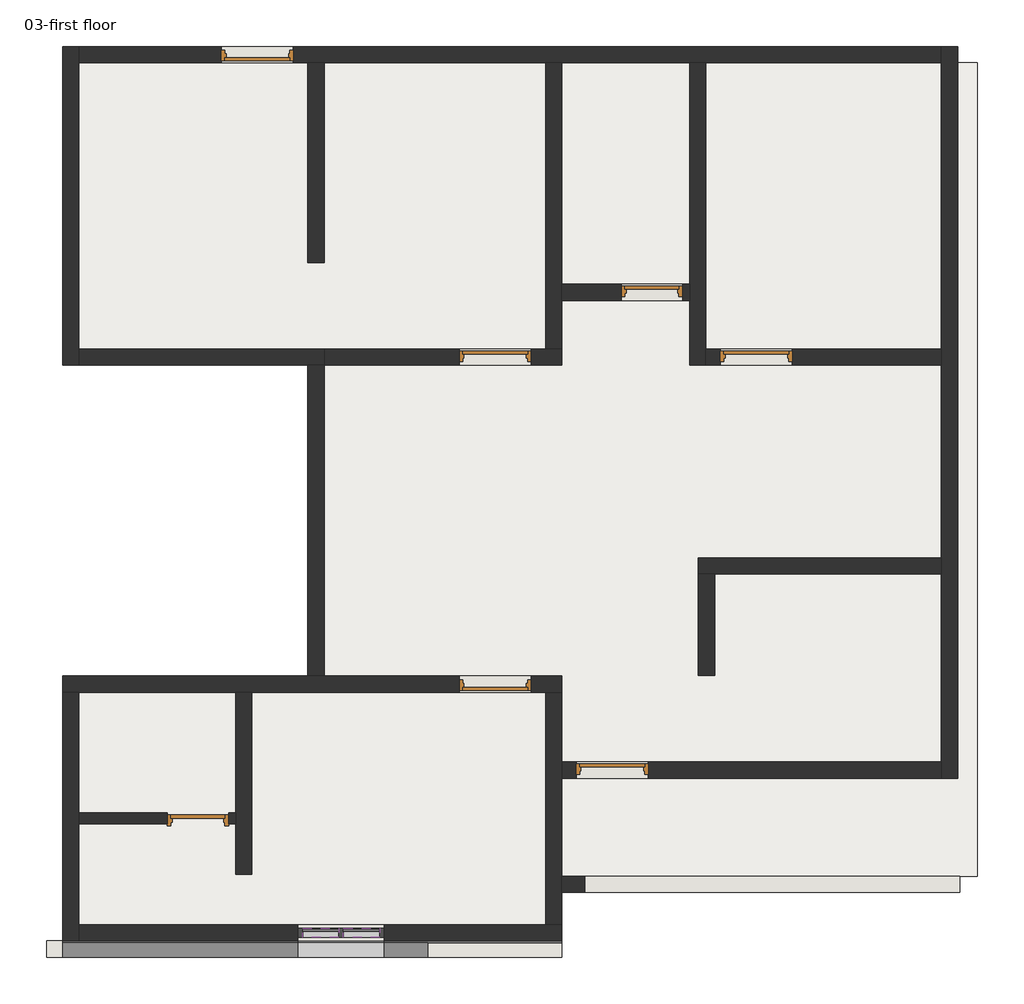
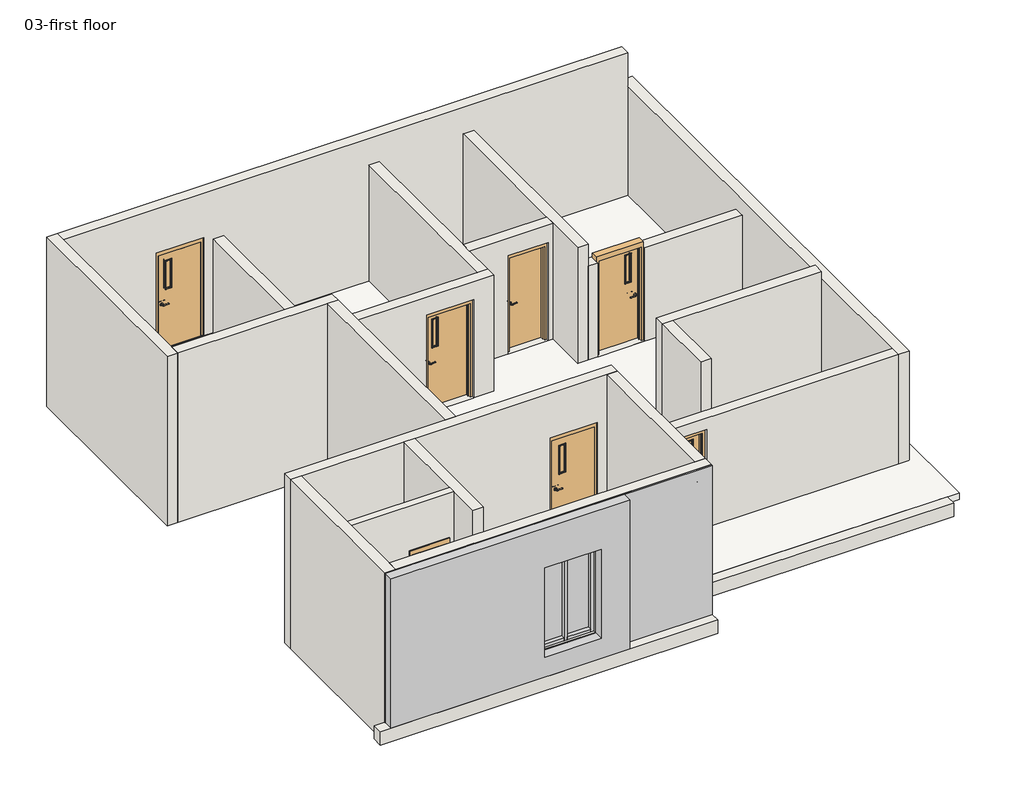
# One storey, incomplete: 23 walls, 7 doors, 7 members, 2 plates, 1 furniture element, 1 slab.
"""IFC4 building model written with IfcOpenShell, lengths in millimetres."""

from ifc_helpers import new_model, si_unit, frame, origin, place, context, project, spatial, polyline, outline, extrude, faceted_brep, transform, mapped, element, save
from components import m_door_passage_single_flush_750_x_2000mm_a9826c90, m_door_passage_single_flush_750_x_2000mm_58848773, m_door_passage_single_vision_lite_900_x_2100_f7eb172f, m_door_passage_single_vision_lite_900_x_2100_15962226, casework_2_casework_2_9c5fcee0, rectangular_mullion_65_x_125mm_rectangular_623ff0e3, rectangular_mullion_65_x_125mm_rectangular_d57ab73f, rectangular_mullion_65_x_125mm_rectangular_2_b62c991d, system_panel_glazed_9cdd2f26

model = new_model("IFC4")

# Units and contexts
model_context = context("Model", 3, world=origin())
ifc_project = project(units=[si_unit("LENGTHUNIT", "METRE", prefix="MILLI")], contexts=[model_context])

# Site, building, storey
site = spatial("IfcSite", under=ifc_project)
building = spatial("IfcBuilding", under=site)
storey = spatial("IfcBuildingStorey", under=building, Name="03-first floor", Elevation=3800.0)

# Doors
placement = place(None, origin())
m_door_passage_single_flush_750_x_2000mm_shape = m_door_passage_single_flush_750_x_2000mm_a9826c90(model_context)
element("IfcDoor", 1, ObjectType="M_Door-Passage-Single-Flush : 750 x 2000mm", at=placement, inside=storey, context=model_context, shape_type="MappedRepresentation", body=[
    mapped(m_door_passage_single_flush_750_x_2000mm_shape, transform((-18812.7520625, -8532.3980844, 4400.0), x_axis=(1.0, 0.0, 0.0), y_axis=(0.0, 1.0, 0.0), z_axis=(0.0, 0.0, 1.0))),
])
m_door_passage_single_flush_750_x_2000mm_2_shape = m_door_passage_single_flush_750_x_2000mm_58848773(model_context)
element("IfcDoor", 2, ObjectType="M_Door-Passage-Single-Flush : 750 x 2000mm", at=placement, inside=storey, context=model_context, shape_type="MappedRepresentation", body=[
    mapped(m_door_passage_single_flush_750_x_2000mm_2_shape, transform((-12512.7520625, -1227.8980844, 4400.0), x_axis=(1.0, 0.0, 0.0), y_axis=(0.0, 1.0, 0.0), z_axis=(0.0, 0.0, 1.0))),
])
m_door_passage_single_vision_lite_900_x_2100_shape = m_door_passage_single_vision_lite_900_x_2100_f7eb172f(model_context)
element("IfcDoor", 3, ObjectType="M_Door-Passage-Single-Vision_Lite : 900 x 2100", at=placement, inside=storey, context=model_context, shape_type="MappedRepresentation", body=[
    mapped(m_door_passage_single_vision_lite_900_x_2100_shape, transform((-13062.7520625, -7859.8980844, 4400.0), x_axis=(-1.0, 0.0, 0.0), y_axis=(0.0, -1.0, 0.0), z_axis=(0.0, 0.0, 1.0))),
])
element("IfcDoor", 4, ObjectType="M_Door-Passage-Single-Vision_Lite : 900 x 2100", at=placement, inside=storey, context=model_context, shape_type="MappedRepresentation", body=[
    mapped(m_door_passage_single_vision_lite_900_x_2100_shape, transform((-11062.7520625, -2127.8980844, 4400.0), x_axis=(-1.0, 0.0, 0.0), y_axis=(0.0, -1.0, 0.0), z_axis=(0.0, 0.0, 1.0))),
])
element("IfcDoor", 5, ObjectType="M_Door-Passage-Single-Vision_Lite : 900 x 2100", at=placement, inside=storey, context=model_context, shape_type="MappedRepresentation", body=[
    mapped(m_door_passage_single_vision_lite_900_x_2100_shape, transform((-14687.7520625, -6655.1980844, 4400.0), x_axis=(1.0, 0.0, 0.0), y_axis=(0.0, 1.0, 0.0), z_axis=(0.0, 0.0, 1.0))),
])
element("IfcDoor", 6, ObjectType="M_Door-Passage-Single-Vision_Lite : 900 x 2100", at=placement, inside=storey, context=model_context, shape_type="MappedRepresentation", body=[
    mapped(m_door_passage_single_vision_lite_900_x_2100_shape, transform((-17987.7520625, 2084.8019156, 4400.0), x_axis=(1.0, 0.0, 0.0), y_axis=(0.0, 1.0, 0.0), z_axis=(0.0, 0.0, 1.0))),
])
m_door_passage_single_vision_lite_900_x_2100_2_shape = m_door_passage_single_vision_lite_900_x_2100_15962226(model_context)
element("IfcDoor", 7, ObjectType="M_Door-Passage-Single-Vision_Lite : 900 x 2100", at=placement, inside=storey, context=model_context, shape_type="MappedRepresentation", body=[
    mapped(m_door_passage_single_vision_lite_900_x_2100_2_shape, transform((-14687.7520625, -2127.8980844, 4400.0), x_axis=(1.0, 0.0, 0.0), y_axis=(0.0, 1.0, 0.0), z_axis=(0.0, 0.0, 1.0))),
])

# Furniture
casework_2_casework_2_shape = casework_2_casework_2_9c5fcee0(model_context)
element("IfcFurniture", 8, ObjectType="Casework 2 : Casework 2", at=placement, inside=storey, context=model_context, shape_type="MappedRepresentation", body=[
    mapped(casework_2_casework_2_shape, transform((0.0, 0.0, 0.0), x_axis=(1.0, 0.0, 0.0), y_axis=(0.0, 1.0, 0.0), z_axis=(0.0, 0.0, 1.0))),
])

# Members
rectangular_mullion_65_x_125mm_rectangular_shape = rectangular_mullion_65_x_125mm_rectangular_623ff0e3(model_context)
element("IfcMember", 9, ObjectType="Rectangular Mullion : 65 x 125mm rectangular", at=placement, inside=storey, context=model_context, shape_type="MappedRepresentation", body=[
    mapped(rectangular_mullion_65_x_125mm_rectangular_shape, transform((-16290.2520625, -10113.5480844, 6700.0), x_axis=(0.0, 0.0, 1.0), y_axis=(0.0, -1.0, 0.0), z_axis=(1.0, 0.0, 0.0))),
])
element("IfcMember", 10, ObjectType="Rectangular Mullion : 65 x 125mm rectangular", at=placement, inside=storey, context=model_context, shape_type="MappedRepresentation", body=[
    mapped(rectangular_mullion_65_x_125mm_rectangular_shape, transform((-16857.7520625, -10113.5480844, 6700.0), x_axis=(0.0, 0.0, 1.0), y_axis=(0.0, -1.0, 0.0), z_axis=(1.0, 0.0, 0.0))),
])
element("IfcMember", 11, ObjectType="Rectangular Mullion : 65 x 125mm rectangular", at=placement, inside=storey, context=model_context, shape_type="MappedRepresentation", body=[
    mapped(rectangular_mullion_65_x_125mm_rectangular_shape, transform((-17360.2520625, -10113.5480844, 4700.0), x_axis=(0.0, 0.0, -1.0), y_axis=(0.0, -1.0, 0.0), z_axis=(-1.0, 0.0, 0.0))),
])
element("IfcMember", 12, ObjectType="Rectangular Mullion : 65 x 125mm rectangular", at=placement, inside=storey, context=model_context, shape_type="MappedRepresentation", body=[
    mapped(rectangular_mullion_65_x_125mm_rectangular_shape, transform((-16792.7520625, -10113.5480844, 4700.0), x_axis=(0.0, 0.0, -1.0), y_axis=(0.0, -1.0, 0.0), z_axis=(-1.0, 0.0, 0.0))),
])
rectangular_mullion_65_x_125mm_rectangular_2_shape = rectangular_mullion_65_x_125mm_rectangular_d57ab73f(model_context)
element("IfcMember", 13, ObjectType="Rectangular Mullion : 65 x 125mm rectangular", at=placement, inside=storey, context=model_context, shape_type="MappedRepresentation", body=[
    mapped(rectangular_mullion_65_x_125mm_rectangular_2_shape, transform((-16225.2520625, -10113.5480844, 4700.0), x_axis=(1.0, 0.0, 0.0), y_axis=(0.0, -1.0, 0.0), z_axis=(0.0, 0.0, -1.0))),
])
element("IfcMember", 14, ObjectType="Rectangular Mullion : 65 x 125mm rectangular", at=placement, inside=storey, context=model_context, shape_type="MappedRepresentation", body=[
    mapped(rectangular_mullion_65_x_125mm_rectangular_2_shape, transform((-17425.2520625, -10113.5480844, 6700.0), x_axis=(-1.0, 0.0, 0.0), y_axis=(0.0, -1.0, 0.0), z_axis=(0.0, 0.0, 1.0))),
])
rectangular_mullion_65_x_125mm_rectangular_2_2_shape = rectangular_mullion_65_x_125mm_rectangular_2_b62c991d(model_context)
element("IfcMember", 15, ObjectType="Rectangular Mullion : 65 x 125mm rectangular 2", at=placement, inside=storey, context=model_context, shape_type="MappedRepresentation", body=[
    mapped(rectangular_mullion_65_x_125mm_rectangular_2_2_shape, transform((-16825.2520625, -10113.5480844, 4700.0), x_axis=(1.0, 0.0, 0.0), y_axis=(0.0, -1.0, 0.0), z_axis=(0.0, 0.0, -1.0))),
])

# Plates
system_panel_glazed_shape = system_panel_glazed_9cdd2f26(model_context)
element("IfcPlate", 16, ObjectType="System Panel : Glazed", at=placement, inside=storey, context=model_context, shape_type="MappedRepresentation", body=[
    mapped(system_panel_glazed_shape, transform((-17109.0020625, -10113.5480844, 4765.0), x_axis=(1.0, 0.0, 0.0), y_axis=(0.0, 1.0, 0.0), z_axis=(0.0, 0.0, 1.0))),
])
element("IfcPlate", 17, ObjectType="System Panel : Glazed", at=placement, inside=storey, context=model_context, shape_type="MappedRepresentation", body=[
    mapped(system_panel_glazed_shape, transform((-16541.5020625, -10113.5480844, 4765.0), x_axis=(1.0, 0.0, 0.0), y_axis=(0.0, 1.0, 0.0), z_axis=(0.0, 0.0, 1.0))),
])

# Slab
element("IfcSlab", 18, ObjectType="01-150 floor", at=placement, inside=storey, context=model_context, shape_type="SweptSolid", body=[
    extrude(outline(polyline([(-7995.7520625, 1965.9519156), (-7995.7520625, -9326.0480844), (-9470.7520625, -9326.0480844), (-13987.7520625, -9326.0480844), (-13987.7520625, -10001.0480844), (-20462.7520625, -10001.0480844), (-20462.7520625, -6774.0480844), (-17062.7520625, -6774.0480844), (-17062.7520625, -2009.0480844), (-20462.7520625, -2009.0480844), (-20462.7520625, 1965.9519156), (-7995.7520625, 1965.9519156)])), frame((0.0, 0.0, 4250.0), z_axis=(0.0, 0.0, 1.0), x_axis=(1.0, 0.0, 0.0)), (0.0, 0.0, 1.0), 150.0),
])

# Walls
element("IfcWall", 19, ObjectType="01-225 wall", at=placement, inside=storey, context=model_context, shape_type="Brep", body=[
    faceted_brep([(-20687.7520625, 2190.9519156, 3800.0), (-20687.7520625, -2234.0480844, 3800.0), (-20687.7520625, -2234.0480844, 7600.0), (-20687.7520625, 2190.9519156, 7600.0), (-20462.7520625, 2190.9519156, 3800.0), (-20462.7520625, 2190.9519156, 7600.0), (-20462.7520625, 1965.9519156, 7600.0), (-20462.7520625, -2009.0480844, 7600.0), (-20462.7520625, -2234.0480844, 7600.0), (-20462.7520625, -2234.0480844, 3800.0), (-20462.7520625, -2009.0480844, 3800.0), (-20462.7520625, 1965.9519156, 3800.0)], [[[0, 1, 2, 3]], [[4, 5, 6, 7, 8, 9, 10, 11]], [[1, 0, 4, 11, 10, 9]], [[3, 2, 8, 7, 6, 5]], [[0, 3, 5, 4]], [[2, 1, 9, 8]]]),
])
element("IfcWall", 20, ObjectType="01-225 wall", at=placement, inside=storey, context=model_context, shape_type="Brep", body=[
    faceted_brep([(-20462.7520625, -10226.0480844, 3800.0), (-13762.7520625, -10226.0480844, 3800.0), (-13762.7520625, -10226.0480844, 7600.0), (-20462.7520625, -10226.0480844, 7600.0), (-17425.2520625, -10226.0480844, 4700.0), (-17425.2520625, -10226.0480844, 6700.0), (-16225.2520625, -10226.0480844, 6700.0), (-16225.2520625, -10226.0480844, 4700.0), (-13762.7520625, -10001.0480844, 3800.0), (-13987.7520625, -10001.0480844, 3800.0), (-20462.7520625, -10001.0480844, 3800.0), (-20462.7520625, -10001.0480844, 7600.0), (-13987.7520625, -10001.0480844, 7600.0), (-13762.7520625, -10001.0480844, 7600.0), (-17425.2520625, -10001.0480844, 6700.0), (-17425.2520625, -10001.0480844, 4700.0), (-16225.2520625, -10001.0480844, 4700.0), (-16225.2520625, -10001.0480844, 6700.0)], [[[0, 1, 2, 3], [4, 5, 6, 7]], [[8, 9, 10, 11, 12, 13], [14, 15, 16, 17]], [[1, 0, 10, 9, 8]], [[3, 2, 13, 12, 11]], [[4, 15, 14, 5]], [[5, 14, 17, 6]], [[6, 17, 16, 7]], [[15, 4, 7, 16]], [[1, 8, 13, 2]], [[3, 11, 10, 0]]]),
])
element("IfcWall", 21, ObjectType="01-225 wall", at=placement, inside=storey, context=model_context, shape_type="Brep", body=[
    faceted_brep([(-8270.7520625, -7966.0480844, 3800.0), (-8270.7520625, 2190.9519156, 3800.0), (-8270.7520625, 2190.9519156, 6850.0), (-8270.7520625, -7966.0480844, 6850.0), (-8495.7520625, -7966.0480844, 3800.0), (-8495.7520625, -7966.0480844, 6850.0), (-8495.7520625, -7741.0480844, 6850.0), (-8495.7520625, 2190.9519156, 6850.0), (-8495.7520625, 2190.9519156, 3800.0), (-8495.7520625, 1965.9519156, 3800.0), (-8495.7520625, -2009.0480844, 3800.0), (-8495.7520625, -2234.0480844, 3800.0), (-8495.7520625, -4909.0480844, 3800.0), (-8495.7520625, -5134.0480844, 3800.0), (-8495.7520625, -7741.0480844, 3800.0)], [[[0, 1, 2, 3]], [[4, 5, 6, 7, 8, 9, 10, 11, 12, 13, 14]], [[1, 0, 4, 14, 13, 12, 11, 10, 9, 8]], [[3, 2, 7, 6, 5]], [[2, 1, 8, 7]], [[0, 3, 5, 4]]]),
])
element("IfcWall", 22, ObjectType="01-225 wall", at=placement, inside=storey, context=model_context, shape_type="Brep", body=[
    faceted_brep([(-8495.7520625, 2190.9519156, 3800.0), (-20462.7520625, 2190.9519156, 3800.0), (-20462.7520625, 2190.9519156, 7600.0), (-8495.7520625, 2190.9519156, 7600.0), (-8495.7520625, 2190.9519156, 6850.0), (-17487.7520625, 2190.9519156, 4400.0), (-17487.7520625, 2190.9519156, 6600.0), (-18487.7520625, 2190.9519156, 6600.0), (-18487.7520625, 2190.9519156, 4400.0), (-8495.7520625, 1965.9519156, 3800.0), (-8495.7520625, 1965.9519156, 7600.0), (-20462.7520625, 1965.9519156, 7600.0), (-20462.7520625, 1965.9519156, 3800.0), (-17287.7520625, 1965.9519156, 3800.0), (-17062.7520625, 1965.9519156, 3800.0), (-13987.7520625, 1965.9519156, 3800.0), (-13762.7520625, 1965.9519156, 3800.0), (-11987.7520625, 1965.9519156, 3800.0), (-11762.7520625, 1965.9519156, 3800.0), (-17487.7520625, 1965.9519156, 4400.0), (-18487.7520625, 1965.9519156, 4400.0), (-18487.7520625, 1965.9519156, 6600.0), (-17487.7520625, 1965.9519156, 6600.0)], [[[0, 1, 2, 3, 4], [5, 6, 7, 8]], [[9, 10, 11, 12, 13, 14, 15, 16, 17, 18], [19, 20, 21, 22]], [[1, 0, 9, 18, 17, 16, 15, 14, 13, 12]], [[3, 2, 11, 10]], [[2, 1, 12, 11]], [[0, 4, 3, 10, 9]], [[6, 5, 19, 22]], [[7, 6, 22, 21]], [[8, 7, 21, 20]], [[5, 8, 20, 19]]]),
])
element("IfcWall", 23, ObjectType="01-225 wall", at=placement, inside=storey, context=model_context, shape_type="SweptSolid", body=[
    extrude(outline(polyline([(-17287.7520625, -809.0480844), (-17287.7520625, 1965.9519156), (-17062.7520625, 1965.9519156), (-17062.7520625, -809.0480844), (-17287.7520625, -809.0480844)])), frame((0.0, 0.0, 3800.0), z_axis=(0.0, 0.0, 1.0), x_axis=(1.0, 0.0, 0.0)), (0.0, 0.0, 1.0), 2700.0),
])
element("IfcWall", 24, ObjectType="01-225 wall", at=placement, inside=storey, context=model_context, shape_type="Brep", body=[
    faceted_brep([(-17062.7520625, -2009.0480844, 7600.0), (-17062.7520625, -2009.0480844, 7000.0), (-17062.7520625, -2009.0480844, 3800.0), (-20462.7520625, -2009.0480844, 3800.0), (-20462.7520625, -2009.0480844, 7600.0), (-17062.7520625, -2234.0480844, 3800.0), (-17062.7520625, -2234.0480844, 7000.0), (-17062.7520625, -2234.0480844, 7600.0), (-17287.7520625, -2234.0480844, 7600.0), (-20462.7520625, -2234.0480844, 7600.0), (-20462.7520625, -2234.0480844, 3800.0), (-17287.7520625, -2234.0480844, 3800.0)], [[[0, 1, 2, 3, 4]], [[5, 6, 7, 8, 9, 10, 11]], [[3, 2, 5, 11, 10]], [[0, 4, 9, 8, 7]], [[4, 3, 10, 9]], [[0, 7, 6, 5, 2, 1]]]),
])
element("IfcWall", 25, ObjectType="01-225 wall", at=placement, inside=storey, context=model_context, shape_type="Brep", body=[
    faceted_brep([(-13762.7520625, -6549.0480844, 3800.0), (-17062.7520625, -6549.0480844, 3800.0), (-17287.7520625, -6549.0480844, 3800.0), (-20687.7520625, -6549.0480844, 3800.0), (-20687.7520625, -6549.0480844, 7600.0), (-17287.7520625, -6549.0480844, 7600.0), (-17062.7520625, -6549.0480844, 7600.0), (-13762.7520625, -6549.0480844, 7600.0), (-14187.7520625, -6549.0480844, 4400.0), (-14187.7520625, -6549.0480844, 6600.0), (-15187.7520625, -6549.0480844, 6600.0), (-15187.7520625, -6549.0480844, 4400.0), (-13762.7520625, -6774.0480844, 3800.0), (-13762.7520625, -6774.0480844, 7600.0), (-13987.7520625, -6774.0480844, 7600.0), (-18062.7520625, -6774.0480844, 7600.0), (-18287.7520625, -6774.0480844, 7600.0), (-20462.7520625, -6774.0480844, 7600.0), (-20687.7520625, -6774.0480844, 7600.0), (-20687.7520625, -6774.0480844, 3800.0), (-20462.7520625, -6774.0480844, 3800.0), (-18287.7520625, -6774.0480844, 3800.0), (-18062.7520625, -6774.0480844, 3800.0), (-13987.7520625, -6774.0480844, 3800.0), (-14187.7520625, -6774.0480844, 4400.0), (-15187.7520625, -6774.0480844, 4400.0), (-15187.7520625, -6774.0480844, 6600.0), (-14187.7520625, -6774.0480844, 6600.0)], [[[0, 1, 2, 3, 4, 5, 6, 7], [8, 9, 10, 11]], [[12, 13, 14, 15, 16, 17, 18, 19, 20, 21, 22, 23], [24, 25, 26, 27]], [[3, 2, 1, 0, 12, 23, 22, 21, 20, 19]], [[7, 6, 5, 4, 18, 17, 16, 15, 14, 13]], [[0, 7, 13, 12]], [[9, 8, 24, 27]], [[10, 9, 27, 26]], [[11, 10, 26, 25]], [[8, 11, 25, 24]], [[4, 3, 19, 18]]]),
])
element("IfcWall", 26, ObjectType="01-225 wall", at=placement, inside=storey, context=model_context, shape_type="Brep", body=[
    faceted_brep([(-18287.7520625, -6774.0480844, 3800.0), (-18287.7520625, -9301.0480844, 3800.0), (-18287.7520625, -9301.0480844, 7600.0), (-18287.7520625, -8601.0480844, 7600.0), (-18287.7520625, -8451.0480844, 7600.0), (-18287.7520625, -6774.0480844, 7600.0), (-18062.7520625, -6774.0480844, 3800.0), (-18062.7520625, -6774.0480844, 7600.0), (-18062.7520625, -9301.0480844, 7600.0), (-18062.7520625, -9301.0480844, 3800.0)], [[[0, 1, 2, 3, 4, 5]], [[6, 7, 8, 9]], [[1, 0, 6, 9]], [[2, 1, 9, 8]], [[5, 4, 3, 2, 8, 7]], [[0, 5, 7, 6]]]),
])
element("IfcWall", 27, ObjectType="01-225 wall", at=placement, inside=storey, context=model_context, shape_type="Brep", body=[
    faceted_brep([(-13987.7520625, -6774.0480844, 3800.0), (-13987.7520625, -10001.0480844, 3800.0), (-13987.7520625, -10001.0480844, 7600.0), (-13987.7520625, -6774.0480844, 7600.0), (-13762.7520625, -6774.0480844, 3800.0), (-13762.7520625, -6774.0480844, 7600.0), (-13762.7520625, -10001.0480844, 7600.0), (-13762.7520625, -10001.0480844, 3800.0), (-13762.7520625, -7966.0480844, 3800.0), (-13762.7520625, -7741.0480844, 3800.0)], [[[0, 1, 2, 3]], [[4, 5, 6, 7, 8, 9]], [[1, 0, 4, 9, 8, 7]], [[3, 2, 6, 5]], [[0, 3, 5, 4]], [[1, 7, 6, 2]]]),
])
element("IfcWall", 28, ObjectType="01-225 wall", at=placement, inside=storey, context=model_context, shape_type="Brep", body=[
    faceted_brep([(-8495.7520625, -7741.0480844, 3800.0), (-13762.7520625, -7741.0480844, 3800.0), (-13762.7520625, -7741.0480844, 6850.0), (-8495.7520625, -7741.0480844, 6850.0), (-13562.7520625, -7741.0480844, 4400.0), (-12562.7520625, -7741.0480844, 4400.0), (-12562.7520625, -7741.0480844, 6600.0), (-13562.7520625, -7741.0480844, 6600.0), (-8495.7520625, -7966.0480844, 3800.0), (-8495.7520625, -7966.0480844, 6850.0), (-13762.7520625, -7966.0480844, 6850.0), (-13762.7520625, -7966.0480844, 4250.0), (-13762.7520625, -7966.0480844, 3800.0), (-13562.7520625, -7966.0480844, 4400.0), (-13562.7520625, -7966.0480844, 6600.0), (-12562.7520625, -7966.0480844, 6600.0), (-12562.7520625, -7966.0480844, 4400.0)], [[[0, 1, 2, 3], [4, 5, 6, 7]], [[8, 9, 10, 11, 12], [13, 14, 15, 16]], [[1, 0, 8, 12]], [[3, 2, 10, 9]], [[0, 3, 9, 8]], [[14, 13, 4, 7]], [[15, 14, 7, 6]], [[16, 15, 6, 5]], [[13, 16, 5, 4]], [[1, 12, 11, 10, 2]]]),
])
element("IfcWall", 29, ObjectType="01-225 wall", at=placement, inside=storey, context=model_context, shape_type="Brep", body=[
    faceted_brep([(-8495.7520625, -4909.0480844, 3800.0), (-11867.7520625, -4909.0480844, 3800.0), (-11867.7520625, -4909.0480844, 7000.0), (-8495.7520625, -4909.0480844, 7000.0), (-8495.7520625, -5134.0480844, 3800.0), (-8495.7520625, -5134.0480844, 7000.0), (-11642.7520625, -5134.0480844, 7000.0), (-11867.7520625, -5134.0480844, 7000.0), (-11867.7520625, -5134.0480844, 3800.0), (-11642.7520625, -5134.0480844, 3800.0)], [[[0, 1, 2, 3]], [[4, 5, 6, 7, 8, 9]], [[1, 0, 4, 9, 8]], [[3, 2, 7, 6, 5]], [[0, 3, 5, 4]], [[2, 1, 8, 7]]]),
])
element("IfcWall", 30, ObjectType="01-225 wall", at=placement, inside=storey, context=model_context, shape_type="SweptSolid", body=[
    extrude(outline(polyline([(-11867.7520625, -6541.0480844), (-11867.7520625, -5134.0480844), (-11642.7520625, -5134.0480844), (-11642.7520625, -6541.0480844), (-11867.7520625, -6541.0480844)])), frame((0.0, 0.0, 3800.0), z_axis=(0.0, 0.0, 1.0), x_axis=(1.0, 0.0, 0.0)), (0.0, 0.0, 1.0), 3200.0),
])
element("IfcWall", 31, ObjectType="01-225 wall", at=placement, inside=storey, context=model_context, shape_type="Brep", body=[
    faceted_brep([(-13987.7520625, 1965.9519156, 3800.0), (-13987.7520625, -2009.0480844, 3800.0), (-13987.7520625, -2009.0480844, 7000.0), (-13987.7520625, 1965.9519156, 7000.0), (-13762.7520625, 1965.9519156, 3800.0), (-13762.7520625, 1965.9519156, 7000.0), (-13762.7520625, -1109.0480844, 7000.0), (-13762.7520625, -1334.0480844, 7000.0), (-13762.7520625, -2009.0480844, 7000.0), (-13762.7520625, -2009.0480844, 3800.0), (-13762.7520625, -1334.0480844, 3800.0), (-13762.7520625, -1109.0480844, 3800.0)], [[[0, 1, 2, 3]], [[4, 5, 6, 7, 8, 9, 10, 11]], [[1, 0, 4, 11, 10, 9]], [[3, 2, 8, 7, 6, 5]], [[0, 3, 5, 4]], [[2, 1, 9, 8]]]),
])
element("IfcWall", 32, ObjectType="01-225 wall", at=placement, inside=storey, context=model_context, shape_type="SweptSolid", body=[
    extrude(outline(polyline([(3800.0, -13762.7520625), (3800.0, -11987.7520625), (7000.0, -11987.7520625), (7000.0, -13762.7520625), (3800.0, -13762.7520625)]), holes=[polyline([(4400.0, -12087.7520625), (4400.0, -12937.7520625), (6600.0, -12937.7520625), (6600.0, -12087.7520625), (4400.0, -12087.7520625)])]), frame((0.0, -1334.0480844, 0.0), z_axis=(0.0, 1.0, 0.0), x_axis=(0.0, 0.0, 1.0)), (0.0, 0.0, 1.0), 225.0),
])
element("IfcWall", 33, ObjectType="01-225 wall", at=placement, inside=storey, context=model_context, shape_type="Brep", body=[
    faceted_brep([(-11762.7520625, -2234.0480844, 3800.0), (-11762.7520625, -2009.0480844, 3800.0), (-11762.7520625, 1965.9519156, 3800.0), (-11762.7520625, 1965.9519156, 7000.0), (-11762.7520625, -2234.0480844, 7000.0), (-11762.7520625, -2234.0480844, 6500.0), (-11987.7520625, -2234.0480844, 3800.0), (-11987.7520625, -2234.0480844, 7000.0), (-11987.7520625, -1334.0480844, 7000.0), (-11987.7520625, -1109.0480844, 7000.0), (-11987.7520625, 1965.9519156, 7000.0), (-11987.7520625, 1965.9519156, 3800.0), (-11987.7520625, -1109.0480844, 3800.0), (-11987.7520625, -1334.0480844, 3800.0)], [[[0, 1, 2, 3, 4, 5]], [[6, 7, 8, 9, 10, 11, 12, 13]], [[2, 1, 0, 6, 13, 12, 11]], [[4, 3, 10, 9, 8, 7]], [[3, 2, 11, 10]], [[0, 5, 4, 7, 6]]]),
])
element("IfcWall", 34, ObjectType="01-225 wall", at=placement, inside=storey, context=model_context, shape_type="Brep", body=[
    faceted_brep([(-17062.7520625, -2234.0480844, 3800.0), (-13762.7520625, -2234.0480844, 3800.0), (-13762.7520625, -2234.0480844, 7000.0), (-17062.7520625, -2234.0480844, 7000.0), (-14187.7520625, -2234.0480844, 4400.0), (-15187.7520625, -2234.0480844, 4400.0), (-15187.7520625, -2234.0480844, 6600.0), (-14187.7520625, -2234.0480844, 6600.0), (-17062.7520625, -2009.0480844, 3800.0), (-17062.7520625, -2009.0480844, 7000.0), (-13987.7520625, -2009.0480844, 7000.0), (-13762.7520625, -2009.0480844, 7000.0), (-13762.7520625, -2009.0480844, 3800.0), (-13987.7520625, -2009.0480844, 3800.0), (-14187.7520625, -2009.0480844, 4400.0), (-14187.7520625, -2009.0480844, 6600.0), (-15187.7520625, -2009.0480844, 6600.0), (-15187.7520625, -2009.0480844, 4400.0)], [[[0, 1, 2, 3], [4, 5, 6, 7]], [[8, 9, 10, 11, 12, 13], [14, 15, 16, 17]], [[1, 0, 8, 13, 12]], [[3, 2, 11, 10, 9]], [[0, 3, 9, 8]], [[2, 1, 12, 11]], [[15, 14, 4, 7]], [[16, 15, 7, 6]], [[17, 16, 6, 5]], [[14, 17, 5, 4]]]),
])
element("IfcWall", 35, ObjectType="01-225 wall", at=placement, inside=storey, context=model_context, shape_type="SweptSolid", body=[
    extrude(outline(polyline([(3800.0, -11762.7520625), (3800.0, -8495.7520625), (6500.0, -8495.7520625), (6500.0, -10562.7520625), (4400.0, -10562.7520625), (4400.0, -11562.7520625), (6500.0, -11562.7520625), (6500.0, -11762.7520625), (3800.0, -11762.7520625)])), frame((0.0, -2234.0480844, 0.0), z_axis=(0.0, 1.0, 0.0), x_axis=(0.0, 0.0, 1.0)), (0.0, 0.0, 1.0), 225.0),
])
element("IfcWall", 36, ObjectType="01-225 wall", at=placement, inside=storey, context=model_context, shape_type="SweptSolid", body=[
    extrude(outline(polyline([(-17287.7520625, -6549.0480844), (-17287.7520625, -2234.0480844), (-17062.7520625, -2234.0480844), (-17062.7520625, -6549.0480844), (-17287.7520625, -6549.0480844)])), frame((0.0, 0.0, 3800.0), z_axis=(0.0, 0.0, 1.0), x_axis=(1.0, 0.0, 0.0)), (0.0, 0.0, 1.0), 3800.0),
])
element("IfcWall", 37, ObjectType="01-225 wall", at=placement, inside=storey, context=model_context, shape_type="Brep", body=[
    faceted_brep([(-20687.7520625, -6774.0480844, 3800.0), (-20687.7520625, -10226.0480844, 3800.0), (-20687.7520625, -10226.0480844, 7600.0), (-20687.7520625, -6774.0480844, 7600.0), (-20462.7520625, -6774.0480844, 3800.0), (-20462.7520625, -6774.0480844, 7600.0), (-20462.7520625, -8451.0480844, 7600.0), (-20462.7520625, -8601.0480844, 7600.0), (-20462.7520625, -10001.0480844, 7600.0), (-20462.7520625, -10226.0480844, 7600.0), (-20462.7520625, -10226.0480844, 3800.0), (-20462.7520625, -10001.0480844, 3800.0)], [[[0, 1, 2, 3]], [[4, 5, 6, 7, 8, 9, 10, 11]], [[1, 0, 4, 11, 10]], [[3, 2, 9, 8, 7, 6, 5]], [[0, 3, 5, 4]], [[1, 10, 9, 2]]]),
])
element("IfcWall", 38, ObjectType="01-225 wall", at=placement, inside=storey, context=model_context, shape_type="Brep", body=[
    faceted_brep([(-13762.7520625, -9551.0480844, 4100.0), (-13442.7520625, -9551.0480844, 4100.0), (-13442.7520625, -9551.0480844, 4400.0), (-13442.7520625, -9551.0480844, 7000.0), (-13762.7520625, -9551.0480844, 7000.0), (-13762.7520625, -9326.0480844, 4100.0), (-13762.7520625, -9326.0480844, 7000.0), (-13442.7520625, -9326.0480844, 7000.0), (-13442.7520625, -9326.0480844, 4400.0), (-13442.7520625, -9326.0480844, 4100.0)], [[[0, 1, 2, 3, 4]], [[5, 6, 7, 8, 9]], [[1, 0, 5, 9]], [[3, 2, 1, 9, 8, 7]], [[4, 3, 7, 6]], [[0, 4, 6, 5]]]),
])
element("IfcWall", 39, ObjectType="01-225 wall", at=placement, inside=storey, context=model_context, shape_type="SweptSolid", body=[
    extrude(outline(polyline([(-8242.7520625, -9551.0480844), (-13442.7520625, -9551.0480844), (-13442.7520625, -9326.0480844), (-8242.7520625, -9326.0480844), (-8242.7520625, -9551.0480844)])), frame((0.0, 0.0, 4100.0), z_axis=(0.0, 0.0, 1.0), x_axis=(1.0, 0.0, 0.0)), (0.0, 0.0, 1.0), 300.0),
])
element("IfcWall", 40, ObjectType="01-225 wall", at=placement, inside=storey, context=model_context, shape_type="SweptSolid", body=[
    extrude(outline(polyline([(-13762.7520625, -10451.0480844), (-20912.7520625, -10451.0480844), (-20912.7520625, -10226.0480844), (-13762.7520625, -10226.0480844), (-13762.7520625, -10451.0480844)])), frame((0.0, 0.0, 3950.0), z_axis=(0.0, 0.0, 1.0), x_axis=(1.0, 0.0, 0.0)), (0.0, 0.0, 1.0), 300.0),
])
element("IfcWall", 41, ObjectType="02-150 wall", at=placement, inside=storey, context=model_context, shape_type="SweptSolid", body=[
    extrude(outline(polyline([(7600.0, -18287.7520625), (7600.0, -20462.7520625), (4400.0, -20462.7520625), (4400.0, -19237.7520625), (6600.0, -19237.7520625), (6600.0, -18387.7520625), (4400.0, -18387.7520625), (4400.0, -18287.7520625), (7600.0, -18287.7520625)])), frame((0.0, -8601.0480844, 0.0), z_axis=(0.0, 1.0, 0.0), x_axis=(0.0, 0.0, 1.0)), (0.0, 0.0, 1.0), 150.0),
])

save(model, "model.ifc")

# Revit data of these elements
# Type "M_Door-Passage-Single-Flush : 750 x 2000mm"
#   Type Mark = "35"
#   Assembly Code = "B2030200"
#   Analytic Construction = "Wooden"
#   Thickness = 45 mm
#   Thermal Resistance (R) = 0.455703 (m²·K)/W
#   Swing Angle [instance default] = 90.00°
#   Strike Height = 1000 mm
#   Rough Width [instance default] = 850 mm
#   Rough Height [instance default] = 2200 mm
#   MF Opening Height [instance default] = 100 mm
#   MF Opening Width [instance default] = 100 mm
#   Inset Calculate [instance default] = 105 mm
#   Masonry Inset [instance default] = 25 mm
#   Height = 2100 mm
#   Width = 750 mm
#   Heat Transfer Coefficient (U) = 2.19465 W/(m²·K)
#   Masonry Frame Depth = 150 mm
#   Masonry Frame [instance default] = yes
#   Function = 1
#   Dry Wall Frame [instance default] = no
#   Panel Material = Wood - Birch
#   Frame Material = Metal - Paint Finish - Grey
#   Door Handle Material = Aluminum
#   Visual Light Transmittance = 0
#   Solar Heat Gain Coefficient = 0
#   Wall Closure = (empty or 0)
# Type "M_Door-Passage-Single-Vision_Lite : 900 x 2100"
#   Type Mark = "46"
#   Assembly Code = "B2030100"
#   Analytic Construction = "Wooden"
#   Thickness = 45 mm
#   Thermal Resistance (R) = 0.455703 (m²·K)/W
#   Swing Angle [instance default] = 90.00°
#   Strike Height = 1000 mm
#   Rough Width [instance default] = 1000 mm
#   Rough Height [instance default] = 2200 mm
#   MFOpeningHeight [instance default] = 100 mm
#   MFOpeningWidth [instance default] = 100 mm
#   Inset Calculate [instance default] = 105 mm
#   Masonry Inset [instance default] = 25 mm
#   Height = 2100 mm
#   Width = 900 mm
#   Heat Transfer Coefficient (U) = 2.19465 W/(m²·K)
#   Masonry Frame Depth = 150 mm
#   Masonry Frame [instance default] = yes
#   Function = 1
#   Dry Wall Frame [instance default] = no
#   Panel Material = Wood - Birch
#   Glazing = Glass
#   Glass Stop Material = Metal - Paint Finish - Grey
#   Frame Material = Metal - Paint Finish - Grey
#   Door Handle Material = Aluminum
#   Visual Light Transmittance = 0
#   Solar Heat Gain Coefficient = 0
#   Wall Closure = (empty or 0)
# Type "Rectangular Mullion : 65 x 125mm rectangular"
#   built-in parameter 1007304 = 0.410105 (stored number, unit not read)
#   built-in parameter 1007301 = 0.106627 (stored number, unit not read)
#   built-in parameter 1007300 = 0.106627 (stored number, unit not read)
# Type "Rectangular Mullion : 65 x 125mm rectangular 2"
#   built-in parameter 1007304 = 0.410105 (stored number, unit not read)
#   built-in parameter 1007301 = 0.106627 (stored number, unit not read)
#   built-in parameter 1007300 = 0.106627 (stored number, unit not read)
# Type "System Panel : Glazed"
#   Construction Type Id = "GSP4R"
#   Analytic Construction = "1/8 in Pilkington single glazing"
#   Visual Light Transmittance = 0.9
#   Solar Heat Gain Coefficient = 0.86
#   Heat Transfer Coefficient (U) = 6.7069 W/(m²·K)
#   Define Thermal Properties by = 1
# Type "01-150 floor"
#   Description = "Generic Floor (Material By Category), 12\" thick"
#   Assembly Code = "B1010"
#   Type Mark = "G01"
#   Function = 0
#   Layers, outside or top first: 150 mm no material (function 1)
# Type "01-225 wall"
#   Description = "Generic Wall (Material By Category), 200mm thick"
#   Assembly Code = "B2010"
#   Type Mark = "G06"
#   Layers, outside or top first: 225 mm "01-225 main wall" (function 1)
# Type "02-150 wall"
#   Description = "Generic Wall (Material By Category), 200mm thick"
#   Assembly Code = "B2010"
#   Type Mark = "G06"
#   Layers, outside or top first: 150 mm "01-225 main wall" (function 1)
# Elements 1, 2 (IfcDoor, "M_Door-Passage-Single-Flush : 750 x 2000mm")
#   Swing Angle = 90.00°
#   Rough Width = 850 mm
#   Rough Height = 2200 mm
#   Masonry Inset = 25 mm
#   MF Opening Width = 100 mm
#   MF Opening Height = 100 mm
#   Inset Calculate = 105 mm
#   Masonry Frame = yes
#   Dry Wall Frame = no
#   Phase Created = New Construction
#   Materials on its faces: "Aluminum", "Metal - Paint Finish - Grey", "Wood - Birch"
# Elements 3, 4, 5, 6, 7 (IfcDoor, "M_Door-Passage-Single-Vision_Lite : 900 x 2100")
#   Swing Angle = 90.00°
#   Rough Width = 1000 mm
#   Rough Height = 2200 mm
#   Masonry Inset = 25 mm
#   MFOpeningWidth = 100 mm
#   MFOpeningHeight = 100 mm
#   Inset Calculate = 105 mm
#   Masonry Frame = yes
#   Dry Wall Frame = no
#   Phase Created = New Construction
#   Materials on its faces: "Metal - Paint Finish - Grey", "Aluminum", "Wood - Birch", "Glass"
# Element 8 (IfcFurniture, "Casework 2 : Casework 2")
#   Phase Created = New Construction
#   Materials on its faces: "Wood Door Panel - Birch", "wood ext"
# Elements 9, 10, 11, 12, 13, 14 (IfcMember, "Rectangular Mullion : 65 x 125mm rectangular")
#   Phase Created = New Construction
#   Materials on its faces: "Aluminum"
# Element 15 (IfcMember, "Rectangular Mullion : 65 x 125mm rectangular 2")
#   Phase Created = New Construction
# Elements 16, 17 (IfcPlate, "System Panel : Glazed")
#   Phase Created = New Construction
#   Materials on its faces: "Glass"
# Element 18 (IfcSlab, "01-150 floor")
#   Height Offset From Level = 600 mm
#   Phase Created = New Construction
#   Materials on its faces: "Default Floor"
# Elements 19, 20, 22, 24, 25, 26, 27, 36, 37 (IfcWall, "01-225 wall")
#   Top Offset = 600 mm
#   Base Offset = 0 mm
#   wall height = 3800 mm
#   Phase Created = New Construction
#   Base Constraint = 03-first floor
#   Top Constraint = 05-second floor
#   Materials on its faces: "01-225 main wall"
# Elements 21, 28 (IfcWall, "01-225 wall")
#   Top Offset = -150 mm
#   Base Offset = 0 mm
#   wall height = 3050 mm
#   Phase Created = New Construction
#   Base Constraint = 03-first floor
#   Top Constraint = 05-second floor
#   Materials on its faces: "01-225 main wall"
# Elements 23, 35 (IfcWall, "01-225 wall")
#   Top Offset = -500 mm
#   Base Offset = 0 mm
#   wall height = 2700 mm
#   Phase Created = New Construction
#   Base Constraint = 03-first floor
#   Top Constraint = 05-second floor
#   Materials on its faces: "01-225 main wall"
# Elements 29, 30, 31, 32, 33, 34 (IfcWall, "01-225 wall")
#   Top Offset = 0 mm
#   Base Offset = 0 mm
#   wall height = 3200 mm
#   Phase Created = New Construction
#   Base Constraint = 03-first floor
#   Top Constraint = 05-second floor
#   Materials on its faces: "01-225 main wall"
# Element 38 (IfcWall, "01-225 wall")
#   built-in parameter 1001111 = 300 mm
#   Top Offset = 0 mm
#   Base Offset = 300 mm
#   wall height = 2900 mm
#   Phase Created = New Construction
#   Base Constraint = 03-first floor
#   Top Constraint = 05-second floor
#   Materials on its faces: "01-225 main wall"
# Element 39 (IfcWall, "01-225 wall")
#   built-in parameter 1001111 = 300 mm
#   Top Offset = 0 mm
#   Base Offset = 300 mm
#   Unconnected Height = 300 mm
#   wall height = 300 mm
#   Phase Created = New Construction
#   Base Constraint = 03-first floor
#   Materials on its faces: "01-225 main wall"
# Element 40 (IfcWall, "01-225 wall")
#   built-in parameter 1001111 = 150 mm
#   Top Offset = 0 mm
#   Base Offset = 150 mm
#   Unconnected Height = 300 mm
#   wall height = 300 mm
#   Phase Created = New Construction
#   Base Constraint = 03-first floor
#   Materials on its faces: "01-225 main wall"
# Element 41 (IfcWall, "02-150 wall")
#   built-in parameter 1001111 = 600 mm
#   Top Offset = 600 mm
#   Base Offset = 600 mm
#   wall height = 3200 mm
#   Phase Created = New Construction
#   Base Constraint = 03-first floor
#   Top Constraint = 05-second floor
#   Materials on its faces: "01-225 main wall"
# Materials
#   "Wood - Birch": class "Wood", colour RGB 173 132 96, transparency 0, Cost = 0
#   "Metal - Paint Finish - Grey": class "Paint", colour RGB 178 178 178, transparency 0, Cost = 0
#   "Aluminum": class "Metal", colour RGB 244 245 246, transparency 0, Description = "Aluminum 6061", Cost = 0
#   "Glass": class "Glass", colour RGB 245 245 243, transparency 1, Description = "Soda Lime Glass", Cost = 0
#   "01-225 main wall": class "Generic", colour RGB 244 244 244, transparency 0, Cost = 0
#   "Wood Door Panel - Birch": class "Wood", colour RGB 166 116 52, transparency 0
#   "wood ext": class "Generic", colour RGB 91 21 0, transparency 0, Cost = 0
#   "Default Floor": colour RGB 128 128 128, transparency 0, Cost = 0
